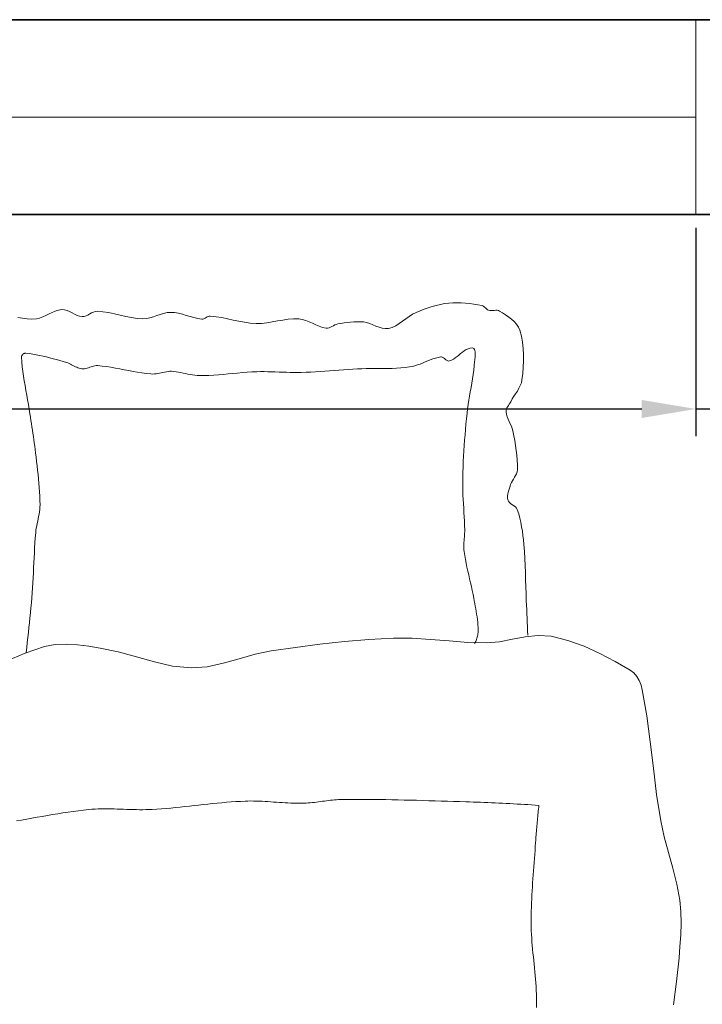
# Model space of a CAD drawing. Units: inches. Extents: x 1484 to 2008, y 1843 to 2590.
# Tile 17 of 21: x 1832 to 1864, y 2172 to 2217. Entities that reach past the tile are written whole.
import ezdxf

# ---------------------------------------------------------------- set-up
doc = ezdxf.new("R2010")
doc.units = ezdxf.units.IN
for name, color, linetype, lineweight in [('A-ANNO-DIMS', 2, 'Continuous', 18), ('A-FURN', 8, 'Continuous', 18), ('A-GLAZ', 4, 'Continuous', 18), ('A-WALL', 7, 'Continuous', 35)]:
    doc.layers.add(name, color=color, linetype=linetype, lineweight=lineweight)
doc.styles.get("Standard").update_dxf_attribs({"font": 'arial.ttf'})
doc.dimstyles.new('ISO-25', dxfattribs={"dimtxt": 7, "dimasz": 2.5, "dimexe": 1.25, "dimexo": 0.625, "dimtad": 1, "dimdec": 0, "dimlunit": 3, "dimtxsty": 'Standard', "dimcen": 2.5, "dimadec": 0, "dimazin": 0, "dimtfac": 1, "dimtdec": 0, "dimtmove": 0, "dimatfit": 3, "dimfxl": 1, "dimarcsym": 0})

# ---------------------------------------------------------------- blocks, each defined once
blk = doc.blocks.new('*D2')
at = {"layer": 'A-ANNO-DIMS', "color": 0, "lineweight": -2, "transparency": 16777216}
for p, q in [((1602.92, 2217.928), (1602.92, 2236.385)), ((1899.92, 2217.928), (1899.92, 2236.385)), ((1605.42, 2235.135), (1897.42, 2235.135))]:
    blk.add_line(p, q, dxfattribs=at)
at = {"layer": 'A-ANNO-DIMS', "color": 0, "transparency": 16777216}
for points in [[(1605.42, 2235.552), (1605.42, 2234.719), (1602.92, 2235.135)], [(1897.42, 2235.552), (1897.42, 2234.719), (1899.92, 2235.135)]]:
    blk.add_solid(points, dxfattribs=at)
at = {"layer": 'Defpoints', "color": 0, "transparency": 16777216}
for p in [(1899.92, 2235.135), (1602.92, 2217.303), (1899.92, 2217.303)]:
    blk.add_point(p, dxfattribs=at)
at = {"layer": 'A-ANNO-DIMS', "color": 0, "transparency": 16777216, "insert": (1750.407, 2239.334), "char_height": 7, "attachment_point": 5}
blk.add_mtext('24\'-9"', dxfattribs=at)
blk = doc.blocks.new('BED-DOUBLE')
for p, q in [((31.278, 84.695), (31.125, 84.673)), ((31.401, 84.686), (31.278, 84.695)), ((31.52, 84.653), (31.401, 84.686)), ((48.027, 84.711), (47.843, 84.64)), ((48.212, 84.777), (48.027, 84.711)), ((48.4, 84.837), (48.212, 84.777)), ((48.589, 84.891), (48.4, 84.837)), ((48.78, 84.936), (48.589, 84.891)), ((48.973, 84.972), (48.78, 84.936)), ((49.167, 84.998), (48.973, 84.972)), ((49.359, 85.013), (49.167, 84.998)), ((49.551, 85.017), (49.359, 85.013)), ((49.744, 85.011), (49.551, 85.017)), ((49.937, 84.997), (49.744, 85.011)), ((50.129, 84.977), (49.937, 84.997)), ((50.321, 84.951), (50.129, 84.977)), ((50.512, 84.921), (50.321, 84.951)), ((50.702, 84.887), (50.512, 84.921)), ((50.746, 84.873), (50.702, 84.887)), ((50.784, 84.848), (50.746, 84.873)), ((50.82, 84.817), (50.784, 84.848)), ((50.855, 84.782), (50.82, 84.817)), ((50.889, 84.745), (50.855, 84.782)), ((50.924, 84.712), (50.889, 84.745)), ((50.962, 84.684), (50.924, 84.712)), ((51.004, 84.664), (50.962, 84.684)), ((29.466, 84.304), (29.252, 84.339)), ((29.68, 84.274), (29.466, 84.304)), ((29.893, 84.259), (29.68, 84.274)), ((30.102, 84.27), (29.893, 84.259)), ((30.254, 84.304), (30.102, 84.27)), ((30.402, 84.358), (30.254, 84.304)), ((30.546, 84.424), (30.402, 84.358)), ((30.689, 84.496), (30.546, 84.424)), ((30.832, 84.567), (30.689, 84.496)), ((30.977, 84.628), (30.832, 84.567)), ((31.125, 84.673), (30.977, 84.628)), ((31.637, 84.603), (31.52, 84.653)), ((31.752, 84.545), (31.637, 84.603)), ((31.867, 84.485), (31.752, 84.545)), ((31.984, 84.431), (31.867, 84.485)), ((32.103, 84.39), (31.984, 84.431)), ((32.226, 84.372), (32.103, 84.39)), ((32.315, 84.379), (32.226, 84.372)), ((32.401, 84.407), (32.315, 84.379)), ((32.485, 84.447), (32.401, 84.407)), ((32.569, 84.494), (32.485, 84.447)), ((32.652, 84.541), (32.569, 84.494)), ((32.736, 84.582), (32.652, 84.541)), ((32.822, 84.61), (32.736, 84.582)), ((32.912, 84.619), (32.822, 84.61)), ((33.179, 84.598), (32.912, 84.619)), ((33.443, 84.556), (33.179, 84.598)), ((33.707, 84.502), (33.443, 84.556)), ((33.97, 84.442), (33.707, 84.502)), ((34.233, 84.382), (33.97, 84.442)), ((34.497, 84.33), (34.233, 84.382)), ((34.762, 84.292), (34.497, 84.33)), ((35.029, 84.275), (34.762, 84.292)), ((35.192, 84.286), (35.029, 84.275)), ((35.352, 84.319), (35.192, 84.286)), ((35.511, 84.366), (35.352, 84.319)), ((35.668, 84.421), (35.511, 84.366)), ((35.826, 84.476), (35.668, 84.421)), ((35.985, 84.524), (35.826, 84.476)), ((36.145, 84.558), (35.985, 84.524)), ((36.307, 84.57), (36.145, 84.558)), ((36.49, 84.557), (36.307, 84.57)), ((36.671, 84.526), (36.49, 84.557)), ((36.85, 84.482), (36.671, 84.526)), ((37.029, 84.43), (36.85, 84.482)), ((37.207, 84.376), (37.029, 84.43)), ((37.386, 84.326), (37.207, 84.376)), ((37.566, 84.285), (37.386, 84.326)), ((37.749, 84.259), (37.566, 84.285)), ((37.8, 84.262), (37.749, 84.259)), ((37.849, 84.277), (37.8, 84.262)), ((37.897, 84.301), (37.849, 84.277)), ((37.945, 84.329), (37.897, 84.301)), ((37.992, 84.357), (37.945, 84.329)), ((38.04, 84.381), (37.992, 84.357)), ((38.09, 84.397), (38.04, 84.381)), ((38.141, 84.4), (38.09, 84.397)), ((38.407, 84.37), (38.141, 84.4)), ((38.672, 84.325), (38.407, 84.37)), ((38.936, 84.272), (38.672, 84.325)), ((39.199, 84.215), (38.936, 84.272)), ((41.737, 84.252), (41.491, 84.216)), ((41.984, 84.272), (41.737, 84.252)), ((42.231, 84.269), (41.984, 84.272)), ((42.394, 84.244), (42.231, 84.269)), ((42.553, 84.197), (42.394, 84.244)), ((47.183, 84.271), (47.031, 84.157)), ((47.337, 84.382), (47.183, 84.271)), ((47.495, 84.483), (47.337, 84.382)), ((47.661, 84.566), (47.495, 84.483)), ((47.843, 84.64), (47.661, 84.566)), ((51.067, 84.651), (51.004, 84.664)), ((51.133, 84.649), (51.067, 84.651)), ((51.2, 84.654), (51.133, 84.649)), ((51.267, 84.661), (51.2, 84.654)), ((51.334, 84.665), (51.267, 84.661)), ((51.398, 84.664), (51.334, 84.665)), ((51.459, 84.653), (51.398, 84.664)), ((51.516, 84.627), (51.459, 84.653)), ((51.654, 84.54), (51.516, 84.627)), ((51.794, 84.449), (51.654, 84.54)), ((51.933, 84.353), (51.794, 84.449)), ((52.065, 84.251), (51.933, 84.353)), ((52.187, 84.141), (52.065, 84.251)), ((39.462, 84.16), (39.199, 84.215)), ((39.726, 84.112), (39.462, 84.16)), ((39.991, 84.075), (39.726, 84.112)), ((40.258, 84.056), (39.991, 84.075)), ((40.506, 84.061), (40.258, 84.056)), ((40.753, 84.087), (40.506, 84.061)), ((40.999, 84.126), (40.753, 84.087)), ((41.245, 84.171), (40.999, 84.126)), ((41.491, 84.216), (41.245, 84.171)), ((42.709, 84.135), (42.553, 84.197)), ((42.863, 84.064), (42.709, 84.135)), ((43.017, 83.992), (42.863, 84.064)), ((43.173, 83.926), (43.017, 83.992)), ((43.331, 83.872), (43.173, 83.926)), ((43.493, 83.838), (43.331, 83.872)), ((43.563, 83.838), (43.493, 83.838)), ((43.631, 83.854), (43.563, 83.838)), ((43.698, 83.881), (43.631, 83.854)), ((43.763, 83.914), (43.698, 83.881)), ((43.829, 83.951), (43.763, 83.914)), ((43.896, 83.986), (43.829, 83.951)), ((43.963, 84.014), (43.896, 83.986)), ((44.033, 84.033), (43.963, 84.014)), ((44.179, 84.057), (44.033, 84.033)), ((44.327, 84.08), (44.179, 84.057)), ((44.475, 84.101), (44.327, 84.08)), ((44.623, 84.118), (44.475, 84.101)), ((44.772, 84.13), (44.623, 84.118)), ((44.92, 84.137), (44.772, 84.13)), ((45.069, 84.136), (44.92, 84.137)), ((45.217, 84.128), (45.069, 84.136)), ((45.365, 84.102), (45.217, 84.128)), ((45.511, 84.056), (45.365, 84.102)), ((45.655, 83.998), (45.511, 84.056)), ((45.799, 83.937), (45.655, 83.998)), ((45.942, 83.881), (45.799, 83.937)), ((46.086, 83.839), (45.942, 83.881)), ((46.231, 83.818), (46.086, 83.839)), ((46.378, 83.826), (46.231, 83.818)), ((46.554, 83.875), (46.378, 83.826)), ((46.719, 83.952), (46.554, 83.875)), ((46.877, 84.048), (46.719, 83.952)), ((47.031, 84.157), (46.877, 84.048)), ((52.294, 84.02), (52.187, 84.141)), ((52.381, 83.888), (52.294, 84.02)), ((52.444, 83.743), (52.381, 83.888)), ((52.52, 83.468), (52.444, 83.743)), ((52.573, 83.186), (52.52, 83.468)), ((49.966, 82.848), (50.055, 82.889)), ((50.055, 82.889), (50.149, 82.915)), ((50.149, 82.915), (50.247, 82.924)), ((50.247, 82.924), (50.294, 82.915)), ((50.294, 82.915), (50.33, 82.891)), ((50.33, 82.891), (50.357, 82.854)), ((52.606, 82.9), (52.573, 83.186)), ((52.621, 82.611), (52.606, 82.9)), ((29.412, 82.499), (29.413, 82.522)), ((29.429, 82.278), (29.412, 82.499)), ((29.413, 82.522), (29.419, 82.546)), ((29.419, 82.546), (29.429, 82.569)), ((29.429, 82.569), (29.443, 82.591)), ((29.443, 82.591), (29.46, 82.612)), ((29.46, 82.612), (29.48, 82.631)), ((29.48, 82.631), (29.502, 82.648)), ((29.502, 82.648), (29.525, 82.662)), ((29.525, 82.662), (29.549, 82.674)), ((29.549, 82.674), (29.574, 82.681)), ((29.574, 82.681), (29.598, 82.685)), ((29.598, 82.685), (29.622, 82.685)), ((29.622, 82.685), (29.781, 82.664)), ((29.781, 82.664), (29.939, 82.639)), ((29.939, 82.639), (30.096, 82.61)), ((30.096, 82.61), (30.253, 82.578)), ((30.253, 82.578), (30.409, 82.543)), ((30.409, 82.543), (30.565, 82.506)), ((30.565, 82.506), (30.721, 82.466)), ((30.721, 82.466), (30.876, 82.425)), ((30.876, 82.425), (31.031, 82.383)), ((48.307, 82.372), (48.426, 82.415)), ((48.426, 82.415), (48.546, 82.454)), ((48.546, 82.454), (48.667, 82.486)), ((48.667, 82.486), (48.791, 82.509)), ((48.791, 82.509), (48.827, 82.509)), ((48.827, 82.509), (48.861, 82.5)), ((48.861, 82.5), (48.895, 82.483)), ((48.895, 82.483), (48.928, 82.461)), ((48.928, 82.461), (48.96, 82.435)), ((48.96, 82.435), (48.992, 82.408)), ((48.992, 82.408), (49.024, 82.381)), ((49.286, 82.356), (49.376, 82.405)), ((49.376, 82.405), (49.463, 82.463)), ((49.463, 82.463), (49.548, 82.528)), ((49.548, 82.528), (49.631, 82.597)), ((49.631, 82.597), (49.713, 82.667)), ((49.713, 82.667), (49.796, 82.734)), ((49.796, 82.734), (49.88, 82.795)), ((49.88, 82.795), (49.966, 82.848)), ((50.357, 82.854), (50.374, 82.807)), ((50.373, 82.419), (50.367, 82.357)), ((50.38, 82.486), (50.373, 82.419)), ((50.374, 82.807), (50.385, 82.751)), ((50.386, 82.555), (50.38, 82.486)), ((50.385, 82.751), (50.39, 82.689)), ((50.39, 82.623), (50.386, 82.555)), ((50.39, 82.689), (50.39, 82.623)), ((52.62, 82.321), (52.621, 82.611)), ((29.452, 82.058), (29.429, 82.278)), ((29.48, 81.839), (29.452, 82.058)), ((31.031, 82.383), (31.186, 82.34)), ((31.186, 82.34), (31.34, 82.296)), ((31.34, 82.296), (31.494, 82.253)), ((31.494, 82.253), (31.556, 82.233)), ((31.556, 82.233), (31.616, 82.208)), ((31.616, 82.208), (31.675, 82.181)), ((31.675, 82.181), (31.733, 82.151)), ((31.733, 82.151), (31.791, 82.12)), ((31.791, 82.12), (31.849, 82.088)), ((31.849, 82.088), (31.907, 82.058)), ((31.907, 82.058), (31.966, 82.03)), ((31.966, 82.03), (32.025, 82.004)), ((32.025, 82.004), (32.085, 81.983)), ((32.085, 81.983), (32.147, 81.967)), ((32.147, 81.967), (32.21, 81.957)), ((32.21, 81.957), (32.271, 81.955)), ((32.271, 81.955), (32.331, 81.961)), ((32.331, 81.961), (32.392, 81.972)), ((32.392, 81.972), (32.451, 81.989)), ((32.451, 81.989), (32.511, 82.008)), ((32.511, 82.008), (32.571, 82.029)), ((32.571, 82.029), (32.63, 82.05)), ((32.63, 82.05), (32.69, 82.07)), ((32.69, 82.07), (32.75, 82.087)), ((32.75, 82.087), (32.81, 82.1)), ((32.81, 82.1), (32.871, 82.107)), ((32.871, 82.107), (32.932, 82.106)), ((32.932, 82.106), (33.138, 82.087)), ((33.138, 82.087), (33.345, 82.061)), ((33.345, 82.061), (33.55, 82.029)), ((33.55, 82.029), (33.755, 81.994)), ((33.755, 81.994), (33.96, 81.955)), ((33.96, 81.955), (34.164, 81.915)), ((44.732, 81.942), (44.948, 81.954)), ((44.948, 81.954), (45.149, 81.962)), ((45.149, 81.962), (45.349, 81.967)), ((45.349, 81.967), (45.55, 81.969)), ((45.55, 81.969), (45.751, 81.97)), ((45.751, 81.97), (45.952, 81.971)), ((45.952, 81.971), (46.153, 81.972)), ((46.153, 81.972), (46.354, 81.975)), ((46.354, 81.975), (46.554, 81.98)), ((46.554, 81.98), (46.754, 81.989)), ((46.754, 81.989), (46.954, 82.002)), ((46.954, 82.002), (47.153, 82.02)), ((47.153, 82.02), (47.352, 82.046)), ((47.352, 82.046), (47.476, 82.068)), ((47.476, 82.068), (47.597, 82.1)), ((47.597, 82.1), (47.717, 82.138)), ((47.717, 82.138), (47.836, 82.181)), ((47.836, 82.181), (47.954, 82.228)), ((47.954, 82.228), (48.072, 82.276)), ((48.072, 82.276), (48.189, 82.325)), ((48.189, 82.325), (48.307, 82.372)), ((49.024, 82.381), (49.057, 82.357)), ((49.057, 82.357), (49.089, 82.336)), ((49.089, 82.336), (49.122, 82.323)), ((49.122, 82.323), (49.156, 82.317)), ((49.156, 82.317), (49.191, 82.321)), ((49.191, 82.321), (49.286, 82.356)), ((50.343, 82.099), (50.319, 81.899)), ((50.361, 82.3), (50.343, 82.099)), ((50.367, 82.357), (50.361, 82.3)), ((52.581, 81.741), (52.606, 82.03)), ((52.606, 82.03), (52.62, 82.321)), ((29.511, 81.62), (29.48, 81.839)), ((29.545, 81.401), (29.511, 81.62)), ((34.164, 81.915), (34.369, 81.875)), ((34.369, 81.875), (34.573, 81.836)), ((34.573, 81.836), (34.778, 81.8)), ((34.778, 81.8), (34.983, 81.768)), ((34.983, 81.768), (35.189, 81.741)), ((35.189, 81.741), (35.396, 81.722)), ((35.396, 81.722), (35.476, 81.719)), ((35.476, 81.719), (35.555, 81.723)), ((35.555, 81.723), (35.635, 81.732)), ((35.635, 81.732), (35.714, 81.745)), ((35.714, 81.745), (35.793, 81.76)), ((35.793, 81.76), (35.872, 81.777)), ((35.872, 81.777), (35.952, 81.795)), ((35.952, 81.795), (36.031, 81.811)), ((36.031, 81.811), (36.11, 81.826)), ((36.11, 81.826), (36.19, 81.837)), ((36.19, 81.837), (36.269, 81.843)), ((36.269, 81.843), (36.349, 81.844)), ((36.349, 81.844), (36.458, 81.837)), ((36.458, 81.837), (36.565, 81.824)), ((36.565, 81.824), (36.673, 81.806)), ((36.673, 81.806), (36.78, 81.786)), ((36.78, 81.786), (36.887, 81.763)), ((36.887, 81.763), (36.994, 81.739)), ((36.994, 81.739), (37.101, 81.716)), ((37.101, 81.716), (37.208, 81.694)), ((37.208, 81.694), (37.315, 81.674)), ((37.315, 81.674), (37.423, 81.659)), ((37.423, 81.659), (37.531, 81.648)), ((37.531, 81.648), (37.639, 81.644)), ((37.639, 81.644), (37.86, 81.646)), ((37.86, 81.646), (38.081, 81.654)), ((38.081, 81.654), (38.302, 81.667)), ((38.302, 81.667), (38.523, 81.683)), ((38.523, 81.683), (38.743, 81.702)), ((38.743, 81.702), (38.964, 81.722)), ((38.964, 81.722), (39.184, 81.743)), ((39.184, 81.743), (39.405, 81.764)), ((39.405, 81.764), (39.625, 81.784)), ((39.625, 81.784), (39.846, 81.801)), ((39.846, 81.801), (40.067, 81.815)), ((40.067, 81.815), (40.288, 81.824)), ((40.288, 81.824), (40.46, 81.828)), ((40.46, 81.828), (40.631, 81.828)), ((40.631, 81.828), (40.803, 81.825)), ((40.803, 81.825), (40.975, 81.821)), ((40.975, 81.821), (41.147, 81.815)), ((41.147, 81.815), (41.318, 81.809)), ((41.318, 81.809), (41.49, 81.802)), ((41.49, 81.802), (41.662, 81.797)), ((41.662, 81.797), (41.834, 81.792)), ((41.834, 81.792), (42.005, 81.789)), ((42.005, 81.789), (42.177, 81.789)), ((42.177, 81.789), (42.349, 81.792)), ((42.349, 81.792), (42.566, 81.799)), ((42.566, 81.799), (42.782, 81.809)), ((42.782, 81.809), (42.999, 81.821)), ((42.999, 81.821), (43.216, 81.835)), ((43.216, 81.835), (43.432, 81.85)), ((43.432, 81.85), (43.649, 81.866)), ((43.649, 81.866), (43.865, 81.882)), ((43.865, 81.882), (44.082, 81.898)), ((44.082, 81.898), (44.298, 81.914)), ((44.298, 81.914), (44.515, 81.928)), ((44.515, 81.928), (44.732, 81.942)), ((50.26, 81.499), (50.226, 81.3)), ((50.291, 81.699), (50.26, 81.499)), ((50.319, 81.899), (50.291, 81.699)), ((52.549, 81.455), (52.581, 81.741)), ((29.582, 81.182), (29.545, 81.401)), ((29.62, 80.964), (29.582, 81.182)), ((50.192, 81.1), (50.157, 80.901)), ((50.226, 81.3), (50.192, 81.1)), ((52.335, 80.933), (52.409, 81.057)), ((52.409, 81.057), (52.472, 81.185)), ((52.472, 81.185), (52.52, 81.317)), ((52.52, 81.317), (52.549, 81.455)), ((29.659, 80.746), (29.62, 80.964)), ((29.698, 80.527), (29.659, 80.746)), ((50.122, 80.702), (50.089, 80.503)), ((50.157, 80.901), (50.122, 80.702)), ((52.099, 80.564), (52.176, 80.687)), ((52.176, 80.687), (52.256, 80.81)), ((52.256, 80.81), (52.335, 80.933)), ((29.736, 80.309), (29.698, 80.527)), ((29.772, 80.09), (29.736, 80.309)), ((50.058, 80.303), (50.031, 80.103)), ((50.089, 80.503), (50.058, 80.303)), ((51.829, 80.094), (51.854, 80.153)), ((51.854, 80.153), (51.887, 80.211)), ((51.887, 80.211), (51.924, 80.267)), ((51.924, 80.267), (51.962, 80.324)), ((51.962, 80.324), (51.998, 80.38)), ((51.998, 80.38), (52.03, 80.437)), ((52.03, 80.437), (52.099, 80.564)), ((29.806, 79.872), (29.772, 80.09)), ((29.828, 79.723), (29.806, 79.872)), ((29.851, 79.574), (29.828, 79.723)), ((50.008, 79.902), (49.983, 79.654)), ((50.031, 80.103), (50.008, 79.902)), ((51.811, 79.971), (51.813, 80.034)), ((51.828, 79.856), (51.811, 79.971)), ((51.813, 80.034), (51.829, 80.094)), ((51.861, 79.744), (51.828, 79.856)), ((51.905, 79.636), (51.861, 79.744)), ((29.874, 79.425), (29.851, 79.574)), ((29.897, 79.276), (29.874, 79.425)), ((29.92, 79.127), (29.897, 79.276)), ((49.959, 79.407), (49.937, 79.159)), ((49.983, 79.654), (49.959, 79.407)), ((51.956, 79.528), (51.905, 79.636)), ((52.008, 79.42), (51.956, 79.528)), ((52.057, 79.312), (52.008, 79.42)), ((52.099, 79.202), (52.057, 79.312)), ((29.943, 78.978), (29.92, 79.127)), ((29.965, 78.829), (29.943, 78.978)), ((29.987, 78.679), (29.965, 78.829)), ((49.915, 78.911), (49.896, 78.663)), ((49.937, 79.159), (49.915, 78.911)), ((52.129, 79.089), (52.099, 79.202)), ((52.172, 78.865), (52.129, 79.089)), ((52.214, 78.64), (52.172, 78.865)), ((30.008, 78.53), (29.987, 78.679)), ((30.027, 78.381), (30.008, 78.53)), ((30.046, 78.231), (30.027, 78.381)), ((49.877, 78.414), (49.861, 78.166)), ((49.896, 78.663), (49.877, 78.414)), ((52.253, 78.415), (52.214, 78.64)), ((52.286, 78.189), (52.253, 78.415)), ((30.063, 78.082), (30.046, 78.231)), ((30.086, 77.881), (30.063, 78.082)), ((30.11, 77.68), (30.086, 77.881)), ((49.846, 77.917), (49.834, 77.669)), ((49.861, 78.166), (49.846, 77.917)), ((52.313, 77.962), (52.286, 78.189)), ((52.332, 77.735), (52.313, 77.962)), ((30.133, 77.479), (30.11, 77.68)), ((30.156, 77.277), (30.133, 77.479)), ((49.823, 77.42), (49.815, 77.172)), ((49.834, 77.669), (49.823, 77.42)), ((52.341, 77.508), (52.332, 77.735)), ((52.337, 77.281), (52.341, 77.508)), ((30.179, 77.076), (30.156, 77.277)), ((30.2, 76.875), (30.179, 77.076)), ((49.815, 77.172), (49.808, 76.923)), ((52.154, 76.863), (52.205, 76.943)), ((52.205, 76.943), (52.254, 77.024)), ((52.254, 77.024), (52.295, 77.106)), ((52.295, 77.106), (52.324, 77.192)), ((52.324, 77.192), (52.337, 77.281)), ((30.219, 76.673), (30.2, 76.875)), ((30.236, 76.472), (30.219, 76.673)), ((49.808, 76.923), (49.807, 76.722)), ((49.807, 76.722), (49.809, 76.522)), ((49.809, 76.522), (49.814, 76.322)), ((51.964, 76.439), (51.995, 76.527)), ((51.995, 76.527), (52.024, 76.614)), ((52.024, 76.614), (52.059, 76.7)), ((52.059, 76.7), (52.103, 76.783)), ((52.103, 76.783), (52.154, 76.863)), ((30.25, 76.27), (30.236, 76.472)), ((30.261, 76.068), (30.25, 76.27)), ((30.268, 75.866), (30.261, 76.068)), ((49.814, 76.322), (49.822, 76.122)), ((49.822, 76.122), (49.831, 75.921)), ((51.877, 76.08), (51.888, 76.17)), ((51.878, 75.991), (51.877, 76.08)), ((51.888, 76.17), (51.908, 76.26)), ((51.908, 76.26), (51.934, 76.35)), ((51.934, 76.35), (51.964, 76.439)), ((30.271, 75.664), (30.268, 75.866)), ((30.268, 75.556), (30.271, 75.664)), ((49.831, 75.921), (49.842, 75.721)), ((49.842, 75.721), (49.854, 75.521)), ((51.893, 75.902), (51.878, 75.991)), ((51.925, 75.833), (51.893, 75.902)), ((51.974, 75.774), (51.925, 75.833)), ((52.037, 75.723), (51.974, 75.774)), ((52.106, 75.675), (52.037, 75.723)), ((52.176, 75.628), (52.106, 75.675)), ((52.241, 75.577), (52.176, 75.628)), ((52.295, 75.519), (52.241, 75.577)), ((30.186, 75.019), (30.208, 75.126)), ((30.208, 75.126), (30.228, 75.233)), ((30.228, 75.233), (30.245, 75.34)), ((30.245, 75.34), (30.259, 75.448)), ((30.259, 75.448), (30.268, 75.556)), ((49.854, 75.521), (49.866, 75.32)), ((49.866, 75.32), (49.877, 75.12)), ((49.877, 75.12), (49.887, 74.92)), ((52.333, 75.452), (52.295, 75.519)), ((52.397, 75.258), (52.333, 75.452)), ((52.45, 75.06), (52.397, 75.258)), ((30.1, 74.59), (30.119, 74.697)), ((30.119, 74.697), (30.14, 74.805)), ((30.14, 74.805), (30.163, 74.912)), ((30.163, 74.912), (30.186, 75.019)), ((49.887, 74.92), (49.895, 74.72)), ((49.895, 74.72), (49.9, 74.519)), ((52.496, 74.861), (52.45, 75.06)), ((52.533, 74.659), (52.496, 74.861)), ((30.052, 74.144), (30.071, 74.374)), ((30.071, 74.374), (30.083, 74.482)), ((30.083, 74.482), (30.1, 74.59)), ((49.893, 74.267), (49.887, 74.183)), ((49.897, 74.351), (49.893, 74.267)), ((49.9, 74.435), (49.897, 74.351)), ((49.9, 74.519), (49.9, 74.435)), ((52.565, 74.456), (52.533, 74.659)), ((52.592, 74.252), (52.565, 74.456)), ((52.615, 74.048), (52.592, 74.252)), ((30.021, 73.682), (30.036, 73.913)), ((30.036, 73.913), (30.052, 74.144)), ((49.863, 73.847), (49.861, 73.764)), ((49.861, 73.764), (49.862, 73.68)), ((49.868, 73.931), (49.863, 73.847)), ((49.873, 74.015), (49.868, 73.931)), ((49.88, 74.099), (49.873, 74.015)), ((49.887, 74.183), (49.88, 74.099)), ((52.635, 73.844), (52.615, 74.048)), ((52.663, 73.518), (52.635, 73.844)), ((29.997, 73.219), (30.009, 73.451)), ((30.009, 73.451), (30.021, 73.682)), ((49.862, 73.68), (49.866, 73.597)), ((49.866, 73.597), (49.875, 73.513)), ((49.875, 73.513), (49.902, 73.331)), ((49.902, 73.331), (49.933, 73.15)), ((52.684, 73.191), (52.663, 73.518)), ((29.976, 72.757), (29.987, 72.988)), ((29.987, 72.988), (29.997, 73.219)), ((49.933, 73.15), (49.968, 72.969)), ((49.968, 72.969), (50.006, 72.789)), ((52.699, 72.864), (52.684, 73.191)), ((52.71, 72.537), (52.699, 72.864)), ((29.953, 72.295), (29.965, 72.526)), ((29.965, 72.526), (29.976, 72.757)), ((50.006, 72.789), (50.046, 72.609)), ((50.046, 72.609), (50.087, 72.429)), ((50.087, 72.429), (50.129, 72.25)), ((52.718, 72.209), (52.71, 72.537)), ((29.925, 71.833), (29.94, 72.063)), ((29.94, 72.063), (29.953, 72.295)), ((50.129, 72.25), (50.171, 72.07)), ((50.171, 72.07), (50.212, 71.891)), ((52.727, 71.882), (52.718, 72.209)), ((29.889, 71.371), (29.908, 71.602)), ((29.908, 71.602), (29.925, 71.833)), ((50.212, 71.891), (50.252, 71.711)), ((50.252, 71.711), (50.289, 71.53)), ((50.289, 71.53), (50.323, 71.349)), ((52.736, 71.554), (52.727, 71.882)), ((52.749, 71.227), (52.736, 71.554)), ((29.849, 70.911), (29.87, 71.141)), ((29.87, 71.141), (29.889, 71.371)), ((50.323, 71.349), (50.345, 71.227)), ((50.345, 71.227), (50.368, 71.104)), ((50.368, 71.104), (50.39, 70.982)), ((52.757, 71.029), (52.749, 71.227)), ((52.766, 70.832), (52.757, 71.029)), ((29.806, 70.451), (29.828, 70.681)), ((29.828, 70.681), (29.849, 70.911)), ((50.39, 70.982), (50.412, 70.859)), ((50.412, 70.859), (50.433, 70.736)), ((50.433, 70.736), (50.453, 70.613)), ((50.453, 70.613), (50.471, 70.49)), ((52.775, 70.634), (52.766, 70.832)), ((52.784, 70.437), (52.775, 70.634)), ((29.76, 69.991), (29.783, 70.221)), ((29.783, 70.221), (29.806, 70.451)), ((50.471, 70.49), (50.488, 70.366)), ((50.488, 70.366), (50.501, 70.243)), ((50.501, 70.243), (50.512, 70.119)), ((50.512, 70.119), (50.52, 69.995)), ((52.793, 70.239), (52.784, 70.437)), ((52.802, 70.042), (52.793, 70.239)), ((29.71, 69.532), (29.735, 69.761)), ((29.735, 69.761), (29.76, 69.991)), ((50.507, 69.658), (50.496, 69.605)), ((50.515, 69.711), (50.507, 69.658)), ((50.521, 69.764), (50.515, 69.711)), ((50.52, 69.995), (50.524, 69.871)), ((50.524, 69.818), (50.521, 69.764)), ((50.524, 69.871), (50.524, 69.818)), ((52.811, 69.844), (52.802, 70.042)), ((52.82, 69.647), (52.811, 69.844)), ((29.657, 69.072), (29.684, 69.302)), ((29.684, 69.302), (29.71, 69.532)), ((30.973, 69.217), (30.471, 69.119)), ((31.488, 69.235), (30.973, 69.217)), ((32.008, 69.198), (31.488, 69.235)), ((43.211, 69.223), (42.083, 69.075)), ((44.342, 69.35), (43.211, 69.223)), ((45.475, 69.449), (44.342, 69.35)), ((46.611, 69.512), (45.475, 69.449)), ((47.469, 69.508), (46.611, 69.512)), ((48.327, 69.451), (47.469, 69.508)), ((49.184, 69.375), (48.327, 69.451)), ((50.042, 69.309), (49.184, 69.375)), ((50.901, 69.287), (50.042, 69.309)), ((50.384, 69.303), (50.358, 69.257)), ((50.408, 69.351), (50.384, 69.303)), ((50.431, 69.4), (50.408, 69.351)), ((50.45, 69.45), (50.431, 69.4)), ((50.468, 69.501), (50.45, 69.45)), ((50.483, 69.552), (50.468, 69.501)), ((50.496, 69.605), (50.483, 69.552)), ((51.502, 69.34), (50.901, 69.287)), ((52.103, 69.452), (51.502, 69.34)), ((52.703, 69.567), (52.103, 69.452)), ((53.299, 69.631), (52.703, 69.567)), ((53.892, 69.59), (53.299, 69.631)), ((54.664, 69.398), (53.892, 69.59)), ((55.416, 69.129), (54.664, 69.398)), ((29.579, 68.813), (28.71, 68.44)), ((30.471, 69.119), (29.579, 68.813)), ((29.629, 68.843), (29.657, 69.072)), ((32.529, 69.128), (32.008, 69.198)), ((33.044, 69.05), (32.529, 69.128)), ((33.889, 68.877), (33.044, 69.05)), ((34.725, 68.644), (33.889, 68.877)), ((40.213, 68.759), (39.476, 68.552)), ((40.957, 68.913), (40.213, 68.759)), ((42.083, 69.075), (40.957, 68.913)), ((56.147, 68.799), (55.416, 69.129)), ((56.86, 68.428), (56.147, 68.799)), ((35.559, 68.405), (34.725, 68.644)), ((36.399, 68.216), (35.559, 68.405)), ((38.741, 68.343), (38.002, 68.186)), ((39.476, 68.552), (38.741, 68.343)), ((57.556, 68.032), (56.86, 68.428)), ((37.252, 68.131), (36.399, 68.216)), ((38.002, 68.186), (37.252, 68.131)), ((57.723, 67.902), (57.556, 68.032)), ((57.861, 67.734), (57.723, 67.902)), ((57.97, 67.541), (57.861, 67.734)), ((58.051, 67.333), (57.97, 67.541)), ((58.105, 67.122), (58.051, 67.333)), ((58.315, 65.917), (58.105, 67.122)), ((58.478, 64.704), (58.315, 65.917)), ((58.621, 63.487), (58.478, 64.704)), ((58.773, 62.272), (58.621, 63.487)), ((39.105, 61.933), (38.89, 61.915)), ((39.32, 61.948), (39.105, 61.933)), ((39.535, 61.96), (39.32, 61.948)), ((39.75, 61.971), (39.535, 61.96)), ((39.882, 61.975), (39.75, 61.971)), ((40.014, 61.976), (39.882, 61.975)), ((40.146, 61.975), (40.014, 61.976)), ((40.277, 61.973), (40.146, 61.975)), ((40.409, 61.968), (40.277, 61.973)), ((40.541, 61.962), (40.409, 61.968)), ((40.673, 61.955), (40.541, 61.962)), ((40.805, 61.946), (40.673, 61.955)), ((40.937, 61.938), (40.805, 61.946)), ((41.069, 61.928), (40.937, 61.938)), ((41.201, 61.919), (41.069, 61.928)), ((41.333, 61.909), (41.201, 61.919)), ((43.045, 61.923), (42.952, 61.912)), ((43.139, 61.936), (43.045, 61.923)), ((43.232, 61.948), (43.139, 61.936)), ((43.326, 61.961), (43.232, 61.948)), ((43.419, 61.973), (43.326, 61.961)), ((43.513, 61.986), (43.419, 61.973)), ((43.606, 61.998), (43.513, 61.986)), ((43.7, 62.009), (43.606, 61.998)), ((43.794, 62.019), (43.7, 62.009)), ((43.887, 62.028), (43.794, 62.019)), ((43.981, 62.036), (43.887, 62.028)), ((44.075, 62.041), (43.981, 62.036)), ((44.169, 62.046), (44.075, 62.041)), ((44.263, 62.048), (44.169, 62.046)), ((44.547, 62.05), (44.263, 62.048)), ((44.832, 62.05), (44.547, 62.05)), ((45.116, 62.05), (44.832, 62.05)), ((45.401, 62.048), (45.116, 62.05)), ((45.685, 62.046), (45.401, 62.048)), ((45.97, 62.042), (45.685, 62.046)), ((46.254, 62.038), (45.97, 62.042)), ((46.538, 62.033), (46.254, 62.038)), ((46.823, 62.027), (46.538, 62.033)), ((47.107, 62.021), (46.823, 62.027)), ((47.392, 62.014), (47.107, 62.021)), ((47.676, 62.007), (47.392, 62.014)), ((47.96, 61.999), (47.676, 62.007)), ((48.245, 61.991), (47.96, 61.999)), ((48.529, 61.982), (48.245, 61.991)), ((48.814, 61.974), (48.529, 61.982)), ((49.098, 61.965), (48.814, 61.974)), ((49.382, 61.956), (49.098, 61.965)), ((49.667, 61.948), (49.382, 61.956)), ((49.951, 61.939), (49.667, 61.948)), ((50.12, 61.934), (49.951, 61.939)), ((50.289, 61.928), (50.12, 61.934)), ((50.459, 61.922), (50.289, 61.928)), ((50.628, 61.916), (50.459, 61.922)), ((50.797, 61.909), (50.628, 61.916)), ((58.961, 61.062), (58.773, 62.272)), ((31.566, 61.462), (31.327, 61.426)), ((31.805, 61.496), (31.566, 61.462)), ((32.045, 61.528), (31.805, 61.496)), ((32.285, 61.556), (32.045, 61.528)), ((32.525, 61.58), (32.285, 61.556)), ((32.671, 61.593), (32.525, 61.58)), ((32.817, 61.602), (32.671, 61.593)), ((32.964, 61.608), (32.817, 61.602)), ((33.11, 61.611), (32.964, 61.608)), ((33.257, 61.613), (33.11, 61.611)), ((33.403, 61.612), (33.257, 61.613)), ((33.55, 61.61), (33.403, 61.612)), ((33.697, 61.607), (33.55, 61.61)), ((33.844, 61.603), (33.697, 61.607)), ((33.991, 61.598), (33.844, 61.603)), ((34.137, 61.593), (33.991, 61.598)), ((34.284, 61.588), (34.137, 61.593)), ((34.431, 61.583), (34.284, 61.588)), ((34.578, 61.579), (34.431, 61.583)), ((34.725, 61.576), (34.578, 61.579)), ((34.872, 61.574), (34.725, 61.576)), ((35.018, 61.574), (34.872, 61.574)), ((35.165, 61.576), (35.018, 61.574)), ((35.312, 61.579), (35.165, 61.576)), ((35.458, 61.586), (35.312, 61.579)), ((35.673, 61.599), (35.458, 61.586)), ((35.888, 61.614), (35.673, 61.599)), ((36.103, 61.631), (35.888, 61.614)), ((36.317, 61.65), (36.103, 61.631)), ((36.532, 61.67), (36.317, 61.65)), ((36.746, 61.692), (36.532, 61.67)), ((36.961, 61.715), (36.746, 61.692)), ((37.175, 61.738), (36.961, 61.715)), ((37.389, 61.762), (37.175, 61.738)), ((37.604, 61.785), (37.389, 61.762)), ((37.818, 61.809), (37.604, 61.785)), ((38.032, 61.832), (37.818, 61.809)), ((38.247, 61.855), (38.032, 61.832)), ((38.461, 61.876), (38.247, 61.855)), ((38.675, 61.897), (38.461, 61.876)), ((38.89, 61.915), (38.675, 61.897)), ((41.465, 61.9), (41.333, 61.909)), ((41.597, 61.892), (41.465, 61.9)), ((41.729, 61.885), (41.597, 61.892)), ((41.861, 61.878), (41.729, 61.885)), ((41.993, 61.873), (41.861, 61.878)), ((42.125, 61.87), (41.993, 61.873)), ((42.257, 61.869), (42.125, 61.87)), ((42.389, 61.87), (42.257, 61.869)), ((42.483, 61.873), (42.389, 61.87)), ((42.577, 61.878), (42.483, 61.873)), ((42.671, 61.884), (42.577, 61.878)), ((42.764, 61.892), (42.671, 61.884)), ((42.858, 61.902), (42.764, 61.892)), ((42.952, 61.912), (42.858, 61.902)), ((50.966, 61.903), (50.797, 61.909)), ((51.135, 61.895), (50.966, 61.903)), ((51.304, 61.888), (51.135, 61.895)), ((51.474, 61.88), (51.304, 61.888)), ((51.643, 61.872), (51.474, 61.88)), ((51.812, 61.864), (51.643, 61.872)), ((51.981, 61.855), (51.812, 61.864)), ((52.15, 61.846), (51.981, 61.855)), ((52.319, 61.837), (52.15, 61.846)), ((52.488, 61.827), (52.319, 61.837)), ((52.657, 61.817), (52.488, 61.827)), ((52.826, 61.807), (52.657, 61.817)), ((52.995, 61.796), (52.826, 61.807)), ((53.164, 61.785), (52.995, 61.796)), ((53.333, 61.774), (53.164, 61.785)), ((53.295, 61.431), (53.304, 61.517)), ((53.304, 61.517), (53.314, 61.603)), ((53.314, 61.603), (53.323, 61.688)), ((53.323, 61.688), (53.333, 61.774)), ((29.421, 61.095), (29.183, 61.054)), ((29.66, 61.136), (29.421, 61.095)), ((29.898, 61.179), (29.66, 61.136)), ((30.136, 61.221), (29.898, 61.179)), ((30.374, 61.264), (30.136, 61.221)), ((30.612, 61.306), (30.374, 61.264)), ((30.85, 61.347), (30.612, 61.306)), ((31.089, 61.387), (30.85, 61.347)), ((31.327, 61.426), (31.089, 61.387)), ((53.253, 61.002), (53.261, 61.088)), ((53.261, 61.088), (53.269, 61.174)), ((53.269, 61.174), (53.278, 61.26)), ((53.278, 61.26), (53.286, 61.345)), ((53.286, 61.345), (53.295, 61.431)), ((59.122, 60.325), (58.961, 61.062)), ((53.208, 60.487), (53.215, 60.573)), ((53.215, 60.573), (53.222, 60.658)), ((53.222, 60.658), (53.229, 60.744)), ((53.229, 60.744), (53.237, 60.83)), ((53.237, 60.83), (53.245, 60.916)), ((53.245, 60.916), (53.253, 61.002)), ((53.177, 60.056), (53.183, 60.142)), ((53.183, 60.142), (53.189, 60.229)), ((53.189, 60.229), (53.195, 60.315)), ((53.195, 60.315), (53.202, 60.401)), ((53.202, 60.401), (53.208, 60.487)), ((59.319, 59.595), (59.122, 60.325)), ((53.137, 59.497), (53.151, 59.684)), ((53.151, 59.684), (53.164, 59.87)), ((53.164, 59.87), (53.177, 60.056)), ((53.109, 59.125), (53.123, 59.311)), ((53.123, 59.311), (53.137, 59.497)), ((59.524, 58.866), (59.319, 59.595)), ((53.067, 58.566), (53.081, 58.752)), ((53.081, 58.752), (53.095, 58.938)), ((53.095, 58.938), (53.109, 59.125)), ((59.707, 58.134), (59.524, 58.866)), ((53.04, 58.193), (53.053, 58.379)), ((53.053, 58.379), (53.067, 58.566)), ((53.006, 57.633), (53.017, 57.82)), ((53.017, 57.82), (53.028, 58.006)), ((53.028, 58.006), (53.04, 58.193)), ((59.842, 57.393), (59.707, 58.134)), ((52.989, 57.26), (52.997, 57.447)), ((52.997, 57.447), (53.006, 57.633)), ((59.89, 56.861), (59.842, 57.393)), ((52.977, 56.887), (52.982, 57.074)), ((52.982, 57.074), (52.989, 57.26)), ((52.971, 56.514), (52.973, 56.701)), ((52.971, 56.327), (52.971, 56.514)), ((52.973, 56.701), (52.977, 56.887)), ((59.901, 56.327), (59.89, 56.861)), ((52.974, 56.154), (52.971, 56.327)), ((52.979, 55.981), (52.974, 56.154)), ((59.883, 55.792), (59.901, 56.327)), ((52.988, 55.808), (52.979, 55.981)), ((52.998, 55.635), (52.988, 55.808)), ((53.011, 55.463), (52.998, 55.635)), ((59.849, 55.256), (59.883, 55.792)), ((53.025, 55.29), (53.011, 55.463)), ((53.041, 55.118), (53.025, 55.29)), ((53.057, 54.945), (53.041, 55.118)), ((59.808, 54.722), (59.849, 55.256)), ((53.075, 54.772), (53.057, 54.945)), ((53.092, 54.6), (53.075, 54.772)), ((59.695, 53.637), (59.808, 54.722)), ((53.11, 54.427), (53.092, 54.6)), ((53.128, 54.255), (53.11, 54.427)), ((53.144, 54.082), (53.128, 54.255)), ((53.161, 53.91), (53.144, 54.082)), ((53.175, 53.737), (53.161, 53.91)), ((53.189, 53.565), (53.175, 53.737)), ((53.2, 53.392), (53.189, 53.565)), ((53.209, 53.219), (53.2, 53.392)), ((59.548, 52.555), (59.695, 53.637)), ((53.216, 53.046), (53.209, 53.219)), ((53.22, 52.873), (53.216, 53.046)), ((53.221, 52.726), (53.22, 52.873)), ((53.216, 52.432), (53.22, 52.579)), ((53.22, 52.579), (53.221, 52.726))]:
    blk.add_line(p, q)
blk = doc.blocks.new('WIN-60IN')
for p, q in [((0, 4.5), (0, -4.5)), ((60, 0), (60, 4.5)), ((60, 4.5), (60, -4.5)), ((0, -4.5), (0, 0)), ((0, 0), (60, 0))]:
    blk.add_line(p, q)
blk = doc.blocks.new('*D13')
at = {"layer": 'A-ANNO-DIMS', "color": 0, "lineweight": -2, "transparency": 16777216}
for p, q in [((1803.22, 2207.678), (1803.22, 2198.053)), ((1863.22, 2207.678), (1863.22, 2198.053)), ((1805.72, 2199.303), (1860.72, 2199.303)), ((1863.22, 2199.303), (2008.197, 2199.303))]:
    blk.add_line(p, q, dxfattribs=at)
at = {"layer": 'A-ANNO-DIMS', "color": 0, "transparency": 16777216}
for points in [[(1805.72, 2199.72), (1805.72, 2198.886), (1803.22, 2199.303)], [(1860.72, 2199.72), (1860.72, 2198.886), (1863.22, 2199.303)]]:
    blk.add_solid(points, dxfattribs=at)
at = {"layer": 'Defpoints', "color": 0, "transparency": 16777216}
for p in [(1803.22, 2208.303), (1863.22, 2208.303), (1863.22, 2199.303)]:
    blk.add_point(p, dxfattribs=at)
at = {"layer": 'A-ANNO-DIMS', "color": 0, "transparency": 16777216, "insert": (1936.959, 2203.55), "char_height": 7, "attachment_point": 5}
blk.add_mtext('BEDROOM WINDOW 5\'-0" TYP.', dxfattribs=at)
blk = doc.blocks.new('*D14')
at = {"layer": 'A-ANNO-DIMS', "color": 0, "lineweight": -2, "transparency": 16777216}
for p, q in [((1872.22, 2217.303), (1872.22, 2263.721)), ((1863.845, 2217.303), (1873.47, 2217.303)), ((1872.22, 2210.803), (1872.22, 2214.803)), ((1863.845, 2208.303), (1873.47, 2208.303))]:
    blk.add_line(p, q, dxfattribs=at)
at = {"layer": 'A-ANNO-DIMS', "color": 0, "transparency": 16777216}
for points in [[(1871.803, 2214.803), (1872.637, 2214.803), (1872.22, 2217.303)], [(1871.803, 2210.803), (1872.637, 2210.803), (1872.22, 2208.303)]]:
    blk.add_solid(points, dxfattribs=at)
at = {"layer": 'Defpoints', "color": 0, "transparency": 16777216}
for p in [(1863.22, 2217.303), (1872.22, 2217.303), (1863.22, 2208.303)]:
    blk.add_point(p, dxfattribs=at)
at = {"layer": 'A-ANNO-DIMS', "color": 0, "transparency": 16777216, "insert": (1868.021, 2241.762), "char_height": 7, "attachment_point": 5, "rotation": 90}
blk.add_mtext('0\'-9" TYP.', dxfattribs=at)

msp = doc.modelspace()

# ---------------------------------------------------------------- linework, layer by layer
at = {"layer": 'A-WALL'}
for p, q in [((1602.92, 2217.303), (1899.92, 2217.303)), ((1602.92, 2217.303), (1899.92, 2217.303)), ((1758.92, 2208.303), (1890.92, 2208.303))]:
    msp.add_line(p, q, dxfattribs=at)

# ---------------------------------------------------------------- block references
at = {"layer": 'A-FURN'}
msp.add_blockref('BED-DOUBLE', (1802.632, 2119.201), dxfattribs=at)
at = {"layer": 'A-GLAZ'}
msp.add_blockref('WIN-60IN', (1803.22, 2212.803), dxfattribs=at)

# ---------------------------------------------------------------- dimensions: what is measured, and where the dimension line sits
at = {"layer": 'A-ANNO-DIMS'}
dim = msp.add_linear_dim(base=(1872.22, 2217.303), p1=(1863.22, 2208.303), p2=(1863.22, 2217.303), angle=90, text='<> TYP.', dimstyle='ISO-25', override={"dimdec": 1, "dimlfac": 1, "dimrnd": 0, "dimzin": 1, "dimdsep": 46, "dimlunit": 4, "dimfrac": 2}, dxfattribs=at)
dim.commit()
dim.dimension.update_dxf_attribs({"geometry": '*D14', "text_midpoint": (1868.021, 2241.762)})
dim = msp.add_linear_dim(base=(1899.92, 2235.135), p1=(1602.92, 2217.303), p2=(1899.92, 2217.303), dimstyle='ISO-25', override={"dimclrd": 0, "dimclre": 0, "dimclrt": 0}, dxfattribs=at)
dim.commit()
dim.dimension.update_dxf_attribs({"geometry": '*D2', "text_midpoint": (1750.407, 2235.135), "dimtype": 160})
dim = msp.add_linear_dim(base=(1863.22, 2199.303), p1=(1803.22, 2208.303), p2=(1863.22, 2208.303), text='BEDROOM WINDOW <> TYP.', dimstyle='ISO-25', override={"dimdec": 1, "dimlfac": 1, "dimrnd": 0, "dimzin": 1, "dimdsep": 46, "dimlunit": 4, "dimfrac": 2}, dxfattribs=at)
dim.commit()
dim.dimension.update_dxf_attribs({"geometry": '*D13', "text_midpoint": (1936.959, 2203.55)})

doc.saveas('drawing.dxf')
